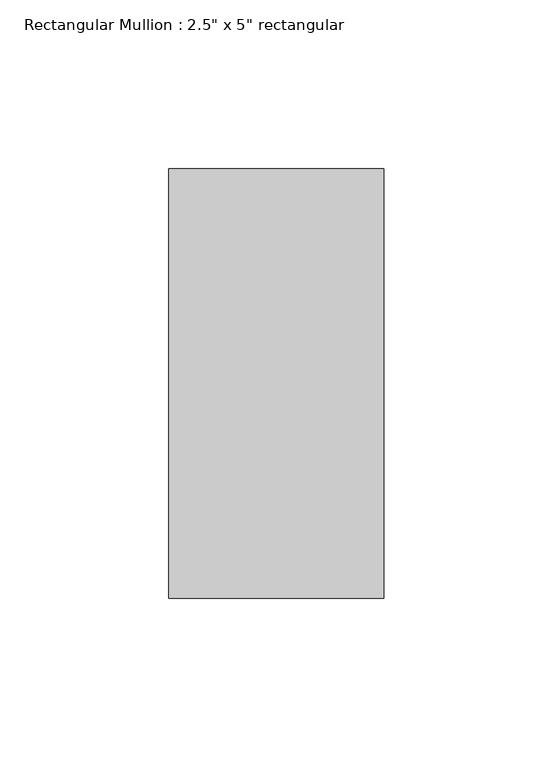
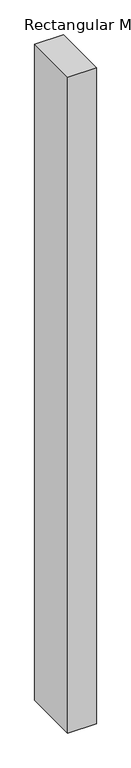
"""IFC4 building model written with IfcOpenShell, lengths in millimetres: member geometry."""

from ifc_helpers import new_model, si_unit, frame, origin, place, context, project, spatial, polyline, outline, extrude, source, transform, mapped, element, save


def member_43b5e5be(model_context):
    return source(origin(), model_context, "Body", "SweptSolid", [
        extrude(outline(polyline([(0.0, 63.5), (0.0, -63.5), (-63.5, -63.5), (-63.5, 63.5), (0.0, 63.5)])), frame((0.0, 0.0, -1538.1940157), z_axis=(0.0, 0.0, 1.0), x_axis=(1.0, 0.0, 0.0)), (0.0, 0.0, 1.0), 1538.1940157),
    ])


if __name__ == "__main__":
    model = new_model("IFC4")
    model_context = context("Model", 3, world=origin())
    ifc_project = project(units=[si_unit("LENGTHUNIT", "METRE", prefix="MILLI")], contexts=[model_context])
    site = spatial("IfcSite", under=ifc_project)
    building = spatial("IfcBuilding", under=site)
    placement = place(None, origin())
    member_shape = member_43b5e5be(model_context)
    element("IfcMember", 1, ObjectType="Rectangular Mullion : 2.5\" x 5\" rectangular", at=placement, inside=building, context=model_context, shape_type="MappedRepresentation", body=[
        mapped(member_shape, transform((0.0, 0.0, 0.0), x_axis=(1.0, 0.0, 0.0), y_axis=(0.0, 1.0, 0.0), z_axis=(0.0, 0.0, 1.0))),
    ])
    save(model, "model.ifc")

# Revit data of these elements
# Type "Rectangular Mullion : 2.5\" x 5\" rectangular"
#   built-in parameter 1007304 = 0.416667 (stored number, unit not read)
#   built-in parameter 1007301 = 0.104167 (stored number, unit not read)
#   built-in parameter 1007300 = 0.104167 (stored number, unit not read)
# Element 1 (IfcMember, "Rectangular Mullion : 2.5\" x 5\" rectangular")
#   Materials on its faces: "Aluminum"
# Materials
#   "Aluminum": class "Metal", colour RGB 247 247 247, transparency 0, Description = "Aluminum 6061", Cost = 0
